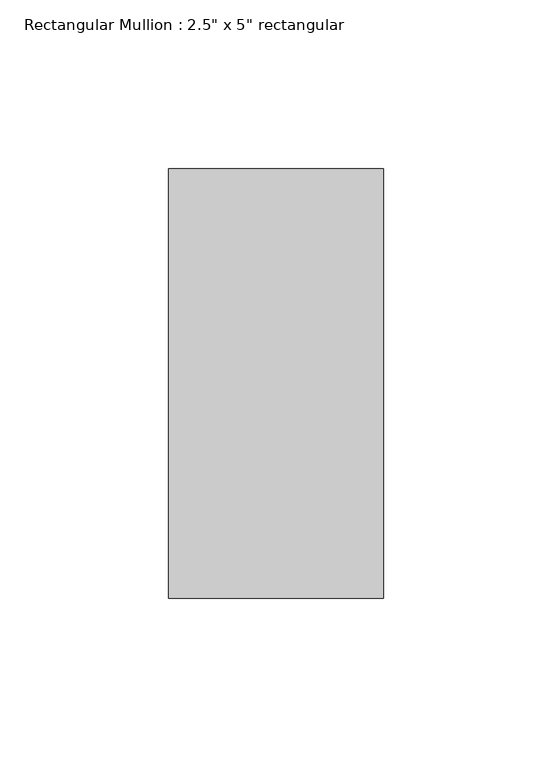
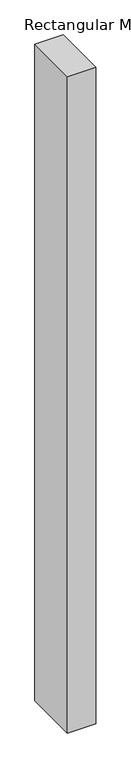
"""IFC4 building model written with IfcOpenShell, lengths in millimetres: member geometry."""

from ifc_helpers import new_model, si_unit, frame, origin, place, context, project, spatial, polyline, outline, extrude, source, transform, mapped, element, save


def member_2edf994d(model_context):
    return source(origin(), model_context, "Body", "SweptSolid", [
        extrude(outline(polyline([(31.75, 63.5), (31.75, -63.5), (-31.75, -63.5), (-31.75, 63.5), (31.75, 63.5)])), frame((0.0, 0.0, -1562.1313909), z_axis=(0.0, 0.0, 1.0), x_axis=(1.0, 0.0, 0.0)), (0.0, 0.0, 1.0), 1562.1313909),
    ])


if __name__ == "__main__":
    model = new_model("IFC4")
    model_context = context("Model", 3, world=origin())
    ifc_project = project(units=[si_unit("LENGTHUNIT", "METRE", prefix="MILLI")], contexts=[model_context])
    site = spatial("IfcSite", under=ifc_project)
    building = spatial("IfcBuilding", under=site)
    placement = place(None, origin())
    member_shape = member_2edf994d(model_context)
    element("IfcMember", 1, ObjectType="Rectangular Mullion : 2.5\" x 5\" rectangular", at=placement, inside=building, context=model_context, shape_type="MappedRepresentation", body=[
        mapped(member_shape, transform((0.0, 0.0, 0.0), x_axis=(1.0, 0.0, 0.0), y_axis=(0.0, 1.0, 0.0), z_axis=(0.0, 0.0, 1.0))),
    ])
    save(model, "model.ifc")

# Revit data of these elements
# Type "Rectangular Mullion : 2.5\" x 5\" rectangular"
#   built-in parameter 1007304 = 0.416667 (stored number, unit not read)
#   built-in parameter 1007301 = 0.104167 (stored number, unit not read)
#   built-in parameter 1007300 = 0.104167 (stored number, unit not read)
# Element 1 (IfcMember, "Rectangular Mullion : 2.5\" x 5\" rectangular")
#   Materials on its faces: "Aluminum"
# Materials
#   "Aluminum": class "Metal", colour RGB 247 247 247, transparency 0, Description = "Aluminum 6061", Cost = 0
